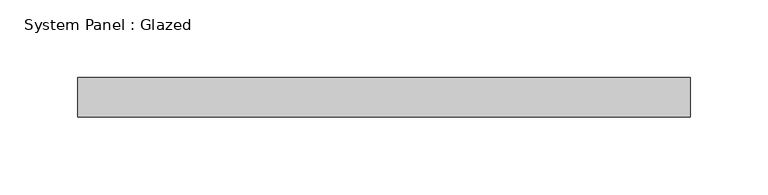
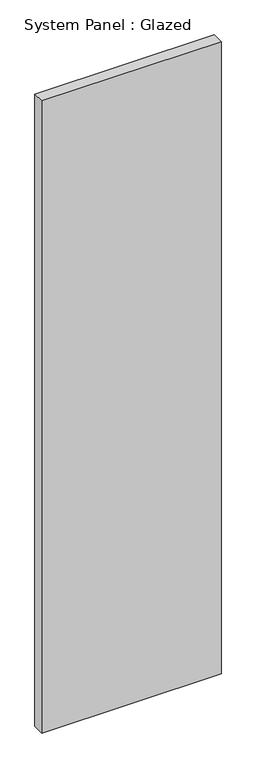
"""IFC4 building model written with IfcOpenShell, lengths in millimetres: plate geometry, System Panel : Glazed."""

from ifc_helpers import new_model, si_unit, origin, origin_with_axes, place, context, project, spatial, polyline, outline, extrude, source, transform, mapped, element, save


def system_panel_glazed_33c81725(model_context):
    return source(origin(), model_context, "Body", "SweptSolid", [
        extrude(outline(polyline([(196.85, 19.05), (-196.85, 19.05), (-196.85, 44.45), (196.85, 44.45), (196.85, 19.05)])), origin_with_axes(), (0.0, 0.0, 1.0), 1466.034917),
    ])


if __name__ == "__main__":
    model = new_model("IFC4")
    model_context = context("Model", 3, world=origin())
    ifc_project = project(units=[si_unit("LENGTHUNIT", "METRE", prefix="MILLI")], contexts=[model_context])
    site = spatial("IfcSite", under=ifc_project)
    building = spatial("IfcBuilding", under=site)
    placement = place(None, origin())
    system_panel_glazed_shape = system_panel_glazed_33c81725(model_context)
    element("IfcPlate", 1, ObjectType="System Panel : Glazed", at=placement, inside=building, context=model_context, shape_type="MappedRepresentation", body=[
        mapped(system_panel_glazed_shape, transform((0.0, 0.0, 0.0), x_axis=(1.0, 0.0, 0.0), y_axis=(0.0, 1.0, 0.0), z_axis=(0.0, 0.0, 1.0))),
    ])
    save(model, "model.ifc")

# Revit data of these elements
# Type "System Panel : Glazed"
#   Construction Type Id = "GSP4R"
#   Analytic Construction = "1/8 in Pilkington single glazing"
#   Visual Light Transmittance = 0.9
#   Solar Heat Gain Coefficient = 0.86
#   Heat Transfer Coefficient (U) = 1.18115 BTU/(h·ft²·°F)
#   Define Thermal Properties by = 1
# Element 1 (IfcPlate, "System Panel : Glazed")
#   Materials on its faces: "Glass"
# Materials
#   "Glass": class "Glass", colour RGB 0 128 192, transparency 0.75, Description = "Soda Lime Glass", Cost = 0
